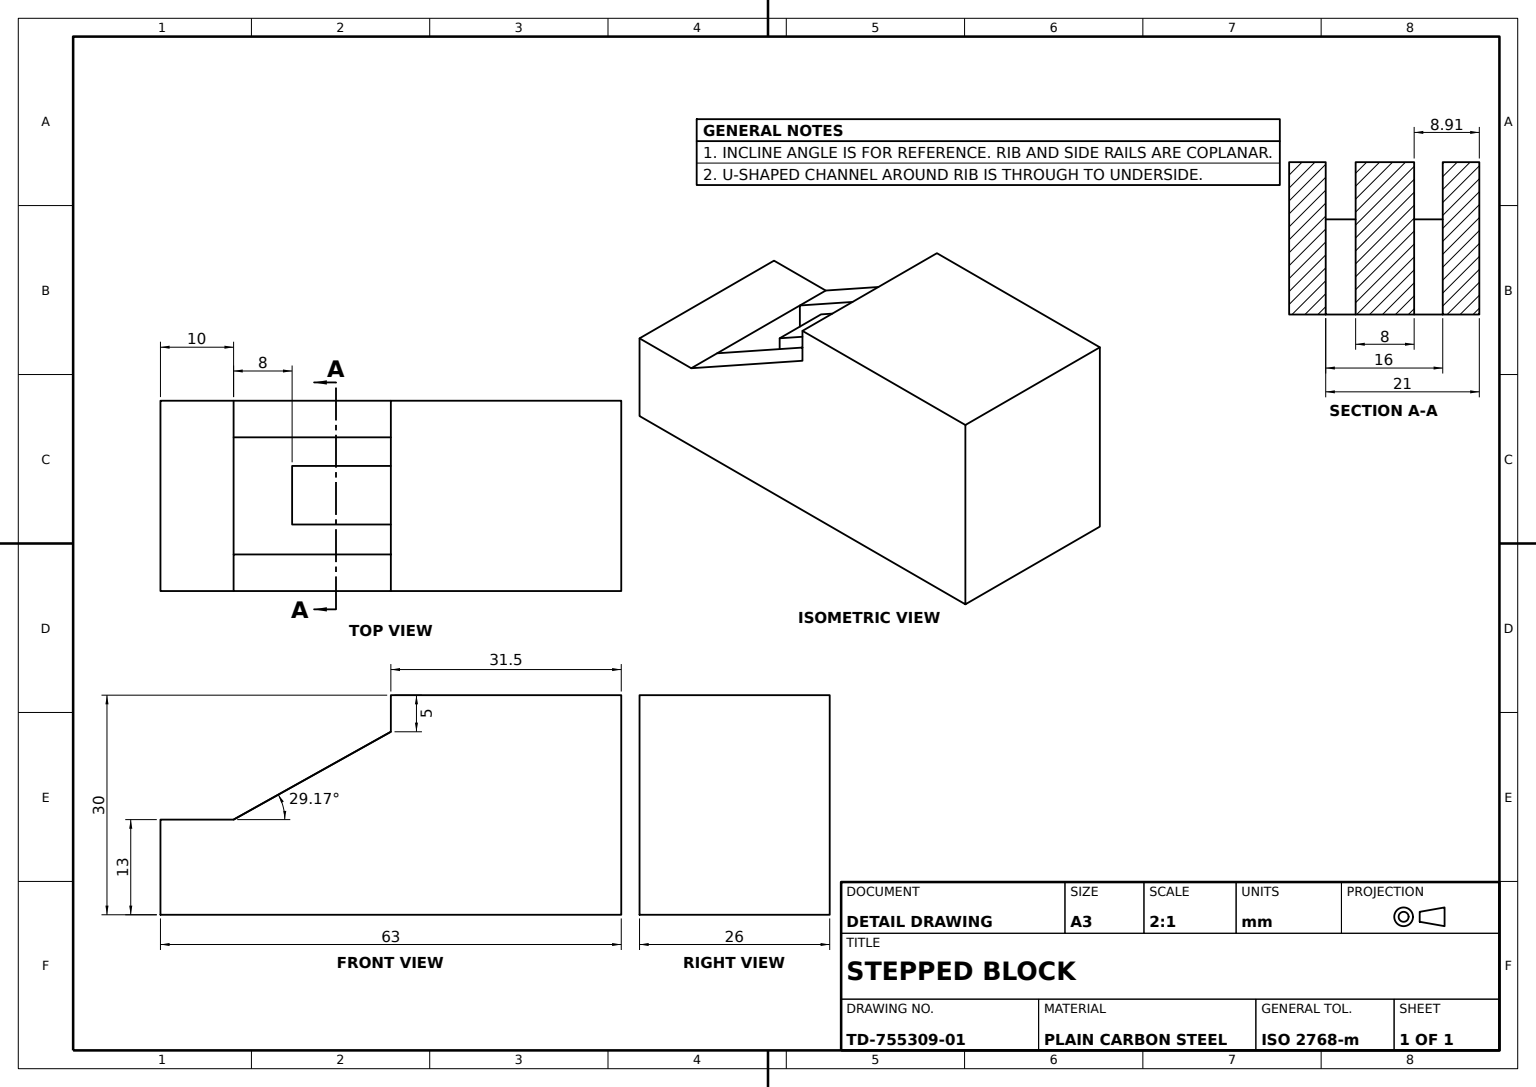
from build123d import *

# Parameters (mm, degrees)
BASE_BLOCK_PROFILE_W       = 63
BASE_BLOCK_PROFILE_H       = 30
BASE_BLOCK_DEPTH           = 26
STEPPED_SLOPE_CUT_DEPTH    = 26
INCLINED_CHANNEL_CUT_DEPTH = 44
CENTRE_RIB_PROFILE_W       = 8
CENTRE_RIB_PROFILE_H       = 25.036205804
CENTRE_RIB_DEPTH           = 30
TOP_NOTCH_CUT_DEPTH        = 30


with BuildPart() as part:
    # Base Block Profile → Base Block (new body)
    with BuildSketch(Plane(origin=(0, 0, 0), x_dir=(0, 0, -1), z_dir=(1, 0, 0))):
        Rectangle(BASE_BLOCK_PROFILE_W, BASE_BLOCK_PROFILE_H)
    extrude(amount=BASE_BLOCK_DEPTH)

    # Stepped Slope Profile → Stepped Slope Cut (cut)
    with BuildSketch(Plane(origin=(26, 0, 0), x_dir=(0, 0, -1), z_dir=(1, 0, 0))):
        Polygon((-31.5, 15), (-31.5, -2), (-21.5, -2), (0, 10), (0, 15), align=None)
    extrude(amount=-STEPPED_SLOPE_CUT_DEPTH, mode=Mode.SUBTRACT)

    # Inclined Channel Profile → Inclined Channel Cut (cut)
    with BuildSketch(Plane(origin=(0, 15, 0), x_dir=(1, 0, 0), z_dir=(0, 1, 0))):
        Polygon((8.908390329, 0), (5, 0), (5, -21.5), (21, -21.5), (21, 0), (16.908390329, 0), (16.908390329, -13.5), (8.908390329, -13.5), align=None)
    extrude(amount=-INCLINED_CHANNEL_CUT_DEPTH, mode=Mode.SUBTRACT)

    # Centre Rib Profile → Centre Rib (add)
    with BuildSketch(Plane.XZ.offset(15)):
        with Locations((12.908390329, 0.981897098)):
            Rectangle(CENTRE_RIB_PROFILE_W, CENTRE_RIB_PROFILE_H)
    extrude(amount=-CENTRE_RIB_DEPTH)

    # Notch Profile → Top Notch Cut (cut)
    with BuildSketch(Plane(origin=(16.908390329, 0, 0), x_dir=(0, 0, -1), z_dir=(1, 0, 0))):
        Polygon((0, 10), (-13.5, 2.465116279), (-13.5, 15), (0, 15), align=None)
    extrude(amount=-TOP_NOTCH_CUT_DEPTH, mode=Mode.SUBTRACT)


solid = part.part
